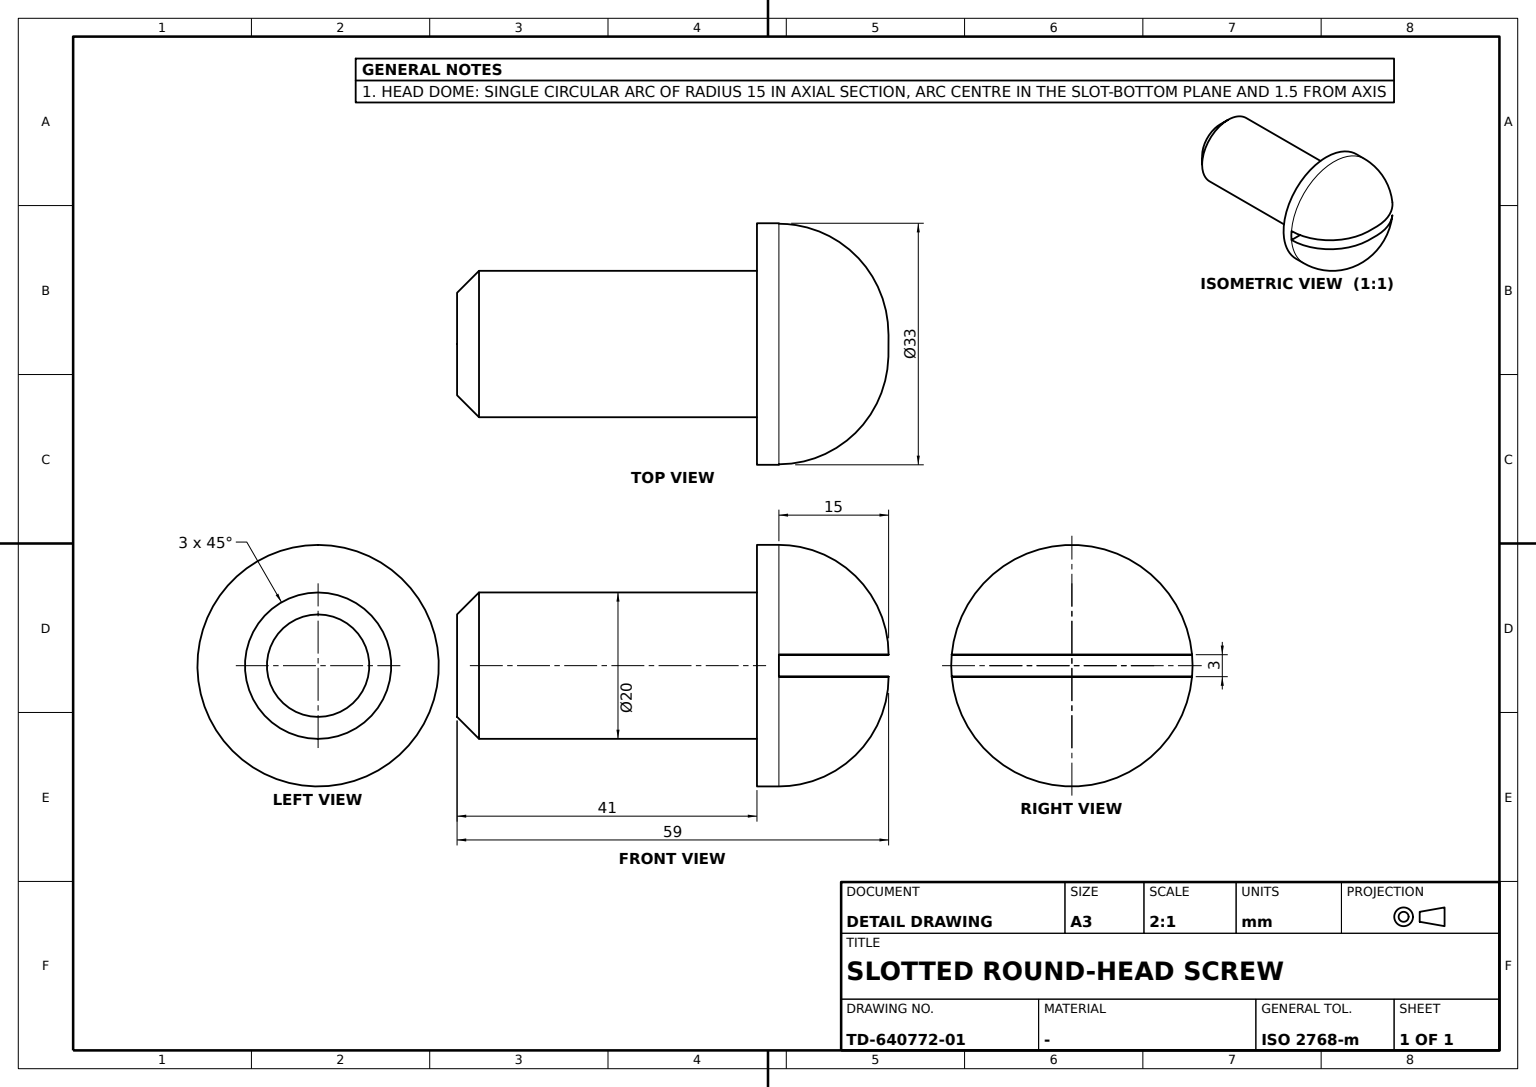
CATIA V5 part; units mm, degrees
sketch "Sketch1" plane through (0, 0, 0) normal (0, 1, 0) x (-1, 0, 0)
  line L0 (0, 0) -> (0, 1.5)
  arc A0 (0, 1.5) -> (15, 16.5) centre (15, 1.5) cw
  line L1 (15, 16.5) -> (18, 16.5)
  line L2 (18, 16.5) -> (18, 10)
  line L3 (18, 10) -> (59, 10)
  line L4 (59, 10) -> (59, 0)
  point P0 (59, 0)
  line L5 (59, 0) -> (0, 0)
  dimension "radius A0" = 15
  dimension "length L4" = 10
  dimension "length L0" = 1.5
  dimension "length L1" = 3
  dimension "distance L2 L4" = 41
  dimension "length L2" = 6.5
  constraint vertical L0 y-axis
  constraint vertical L2 y-axis
  constraint vertical L4 y-axis
  constraint tangency A0 L0
  constraint tangency L1 A0
  constraint horizontal L3 x-axis
  constraint horizontal L5 x-axis
  constraint coincidence P0 x-axis
revolve "Shaft1" add sketch "Sketch1" angle 360 about L5
chamfer "Chamfer1" distance 3 angle 45 1 edges at (-59, 0, -10)
sketch "Sketch2" plane through (0, 0, 0) normal (1, 0, 0) x (0, 1, 0)
  line L0 (16.5, 1.5) -> (16.5, -1.5)
  line L1 (16.5, -1.5) -> (-16.5, -1.5)
  line L2 (-16.5, -1.5) -> (-16.5, 1.5)
  line L3 (-16.5, 1.5) -> (16.5, 1.5)
  dimension "length L3" = 33
  dimension "length L0" = 3
  constraint vertical L0 y-axis
  constraint vertical L2 y-axis
  constraint horizontal L1 x-axis
  constraint horizontal L3 x-axis
  constraint equidistance L0 L2 origin
  constraint equidistance L1 L3 origin
extrude "Pocket1" cut sketch "Sketch2" against normal blind 15
